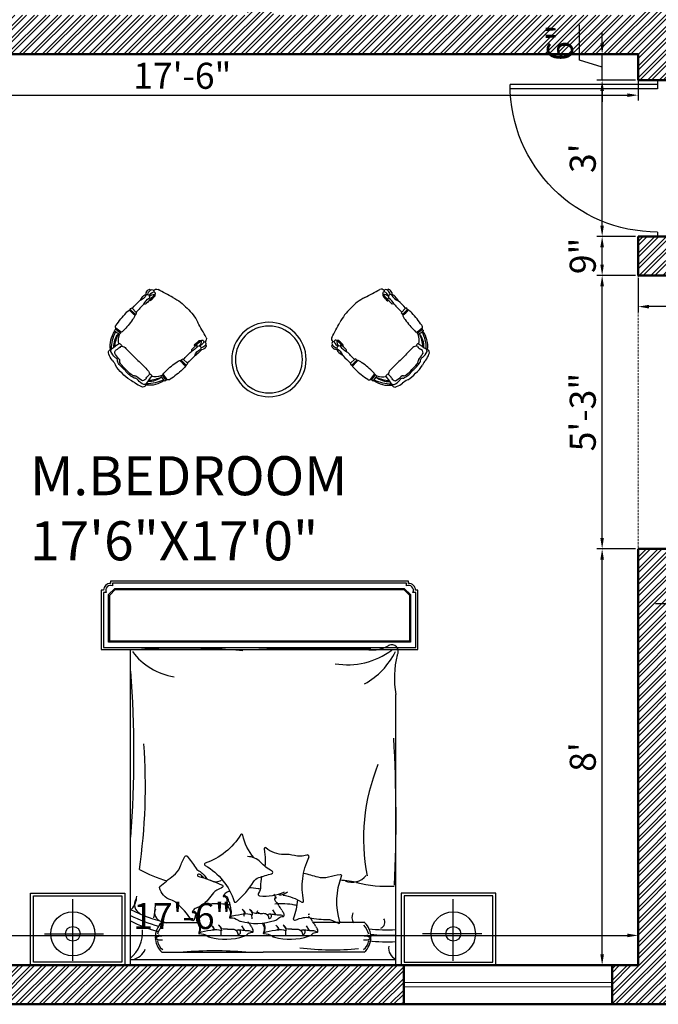
# Model space of a CAD drawing. Units: inches. Extents: x 3590 to 5167, y 65 to 1917.
# Tile 2 of 100: x 3722 to 3869, y 109 to 336. Entities that reach past the tile are written whole.
import ezdxf

# ---------------------------------------------------------------- set-up
doc = ezdxf.new("R2010")
doc.units = ezdxf.units.IN
doc.linetypes.add('DASHED', pattern=[0.75, 0.5, -0.25])
for name, color, linetype, lineweight in [('A-ANNO-DIMS', 2, 'Continuous', 18), ('A-AREA-IDEN', 7, 'Continuous', 18), ('A-DOOR', 3, 'Continuous', 25), ('A-FURN', 21, 'Continuous', 18), ('A-GLAZ', 4, 'Continuous', 18), ('A-WALL', 7, 'Continuous', 50), ('A-WALL-PATT', 251, 'Continuous', 13), ('S-BEAM-OVHD', 7, 'DASHED', 18)]:
    doc.layers.add(name, color=color, linetype=linetype, lineweight=lineweight)
for name, color, linetype in [('FUR', 42, 'Continuous'), ('furn', 7, 'Continuous'), ('HA-FUR', 8, 'Continuous'), ('HA-P', 8, 'Continuous'), ('SAN', 5, 'Continuous'), ('wood', 26, 'Continuous')]:
    doc.layers.add(name, color=color, linetype=linetype)
doc.styles.get("Standard").update_dxf_attribs({"font": 'arial.ttf'})
doc.dimstyles.new('ISO-25', dxfattribs={"dimtxt": 9, "dimasz": 2.5, "dimexe": 1.25, "dimexo": 0.625, "dimtad": 1, "dimdec": 1, "dimlunit": 3, "dimtxsty": 'Standard', "dimcen": 2.5, "dimadec": 0, "dimazin": 0, "dimtfac": 1, "dimtdec": 1, "dimtmove": 0, "dimatfit": 3, "dimfxl": 1, "dimarcsym": 0})

# ---------------------------------------------------------------- blocks, each defined once
blk = doc.blocks.new('D1')
for p, q in [((1, 0), (1, 34)), ((2, 0), (2, 33.99)), ((0, 0), (2, 0)), ((35, 0), (36, 0))]:
    blk.add_line(p, q)
at = {"ltscale": 0.5}
blk.add_arc((1, 0), 34, 0, 90, dxfattribs=at)
blk = doc.blocks.new('*D240')
at = {"layer": 'A-ANNO-DIMS', "color": 0, "lineweight": -2, "transparency": 16777216}
for p, q in [((3654.51, 327.43), (3654.51, 317.35)), ((3864.51, 327.43), (3864.51, 317.35)), ((3657.01, 318.6), (3862.01, 318.6))]:
    blk.add_line(p, q, dxfattribs=at)
at = {"layer": 'A-ANNO-DIMS', "color": 0, "transparency": 16777216}
for points in [[(3657.01, 319.02), (3657.01, 318.18), (3654.51, 318.6)], [(3862.01, 319.02), (3862.01, 318.18), (3864.51, 318.6)]]:
    blk.add_solid(points, dxfattribs=at)
at = {"layer": 'Defpoints', "color": 0, "transparency": 16777216}
for p in [(3654.51, 328.06), (3864.51, 328.06), (3864.51, 318.6)]:
    blk.add_point(p, dxfattribs=at)
at = {"layer": 'A-ANNO-DIMS', "color": 0, "transparency": 16777216, "insert": (3759.51, 322.29), "char_height": 6, "attachment_point": 5}
blk.add_mtext('17\'-6"', dxfattribs=at)
blk = doc.blocks.new('*D194')
at = {"layer": 'A-ANNO-DIMS', "color": 0, "lineweight": -2, "transparency": 16777216}
for p, q in [((3654.51, 118.68), (3654.51, 126.19)), ((3657.01, 124.94), (3862.01, 124.94)), ((3864.51, 118.68), (3864.51, 126.19))]:
    blk.add_line(p, q, dxfattribs=at)
at = {"layer": 'A-ANNO-DIMS', "color": 0, "transparency": 16777216}
for points in [[(3657.01, 125.36), (3657.01, 124.52), (3654.51, 124.94)], [(3862.01, 125.36), (3862.01, 124.52), (3864.51, 124.94)]]:
    blk.add_solid(points, dxfattribs=at)
at = {"layer": 'Defpoints', "color": 0, "transparency": 16777216}
for p in [(3864.51, 124.94), (3654.51, 118.06), (3864.51, 118.06)]:
    blk.add_point(p, dxfattribs=at)
at = {"layer": 'A-ANNO-DIMS', "color": 0, "transparency": 16777216, "insert": (3759.51, 128.63), "char_height": 6, "attachment_point": 5}
blk.add_mtext('17\'-6"', dxfattribs=at)
blk = doc.blocks.new('*D195')
at = {"layer": 'A-ANNO-DIMS', "color": 0, "lineweight": -2, "transparency": 16777216}
for p, q in [((3863.89, 214.06), (3854.98, 214.06)), ((3856.23, 120.56), (3856.23, 211.56)), ((3863.89, 118.06), (3854.98, 118.06))]:
    blk.add_line(p, q, dxfattribs=at)
at = {"layer": 'A-ANNO-DIMS', "color": 0, "transparency": 16777216}
for points in [[(3855.81, 211.56), (3856.64, 211.56), (3856.23, 214.06)], [(3855.81, 120.56), (3856.64, 120.56), (3856.23, 118.06)]]:
    blk.add_solid(points, dxfattribs=at)
at = {"layer": 'Defpoints', "color": 0, "transparency": 16777216}
for p in [(3856.23, 214.06), (3864.51, 214.06), (3864.51, 118.06)]:
    blk.add_point(p, dxfattribs=at)
at = {"layer": 'A-ANNO-DIMS', "color": 0, "transparency": 16777216, "insert": (3852.54, 166.06), "char_height": 6, "attachment_point": 5, "rotation": 90}
blk.add_mtext("8'", dxfattribs=at)
blk = doc.blocks.new('*D196')
at = {"layer": 'A-ANNO-DIMS', "color": 0, "lineweight": -2, "transparency": 16777216}
for p, q in [((3863.89, 277.06), (3854.98, 277.06)), ((3856.23, 216.56), (3856.23, 274.56)), ((3863.89, 214.06), (3854.98, 214.06))]:
    blk.add_line(p, q, dxfattribs=at)
at = {"layer": 'A-ANNO-DIMS', "color": 0, "transparency": 16777216}
for points in [[(3855.81, 274.56), (3856.64, 274.56), (3856.23, 277.06)], [(3855.81, 216.56), (3856.64, 216.56), (3856.23, 214.06)]]:
    blk.add_solid(points, dxfattribs=at)
at = {"layer": 'Defpoints', "color": 0, "transparency": 16777216}
for p in [(3856.23, 277.06), (3864.51, 277.06), (3864.51, 214.06)]:
    blk.add_point(p, dxfattribs=at)
at = {"layer": 'A-ANNO-DIMS', "color": 0, "transparency": 16777216, "insert": (3852.54, 245.56), "char_height": 6, "attachment_point": 5, "rotation": 90}
blk.add_mtext('5\'-3"', dxfattribs=at)
blk = doc.blocks.new('*D197')
at = {"layer": 'A-ANNO-DIMS', "color": 0, "lineweight": -2, "transparency": 16777216}
for p, q in [((3863.89, 286.06), (3854.98, 286.06)), ((3856.23, 279.56), (3856.23, 283.56)), ((3863.89, 277.06), (3854.98, 277.06))]:
    blk.add_line(p, q, dxfattribs=at)
at = {"layer": 'A-ANNO-DIMS', "color": 0, "transparency": 16777216}
for points in [[(3855.81, 283.56), (3856.64, 283.56), (3856.23, 286.06)], [(3855.81, 279.56), (3856.64, 279.56), (3856.23, 277.06)]]:
    blk.add_solid(points, dxfattribs=at)
at = {"layer": 'Defpoints', "color": 0, "transparency": 16777216}
for p in [(3856.23, 286.06), (3864.51, 286.06), (3864.51, 277.06)]:
    blk.add_point(p, dxfattribs=at)
at = {"layer": 'A-ANNO-DIMS', "color": 0, "transparency": 16777216, "insert": (3852.54, 281.56), "char_height": 6, "attachment_point": 5, "rotation": 90}
blk.add_mtext('9"', dxfattribs=at)
blk = doc.blocks.new('*D198')
at = {"layer": 'A-ANNO-DIMS', "color": 0, "lineweight": -2, "transparency": 16777216}
for p, q in [((3863.89, 322.06), (3854.98, 322.06)), ((3856.23, 288.56), (3856.23, 319.56)), ((3863.89, 286.06), (3854.98, 286.06))]:
    blk.add_line(p, q, dxfattribs=at)
at = {"layer": 'A-ANNO-DIMS', "color": 0, "transparency": 16777216}
for points in [[(3855.81, 319.56), (3856.64, 319.56), (3856.23, 322.06)], [(3855.81, 288.56), (3856.64, 288.56), (3856.23, 286.06)]]:
    blk.add_solid(points, dxfattribs=at)
at = {"layer": 'Defpoints', "color": 0, "transparency": 16777216}
for p in [(3856.23, 322.06), (3864.51, 322.06), (3864.51, 286.06)]:
    blk.add_point(p, dxfattribs=at)
at = {"layer": 'A-ANNO-DIMS', "color": 0, "transparency": 16777216, "insert": (3852.54, 304.06), "char_height": 6, "attachment_point": 5, "rotation": 90}
blk.add_mtext("3'", dxfattribs=at)
blk = doc.blocks.new('*D172')
at = {"layer": 'A-ANNO-DIMS', "color": 0, "lineweight": -2, "transparency": 16777216}
for p, q in [((3850.98, 326.64), (3850.98, 334.81)), ((3856.23, 330.56), (3856.23, 333.06)), ((3863.89, 328.06), (3854.98, 328.06)), ((3856.23, 322.06), (3856.23, 328.06)), ((3856.23, 322.06), (3856.23, 328.06)), ((3856.23, 325.06), (3850.98, 326.64)), ((3863.89, 322.06), (3854.98, 322.06)), ((3856.23, 319.56), (3856.23, 317.06))]:
    blk.add_line(p, q, dxfattribs=at)
at = {"layer": 'A-ANNO-DIMS', "color": 0, "transparency": 16777216}
for points in [[(3855.81, 330.56), (3856.64, 330.56), (3856.23, 328.06)], [(3855.81, 319.56), (3856.64, 319.56), (3856.23, 322.06)]]:
    blk.add_solid(points, dxfattribs=at)
at = {"layer": 'Defpoints', "color": 0, "transparency": 16777216}
for p in [(3856.23, 328.06), (3864.51, 328.06), (3864.51, 322.06)]:
    blk.add_point(p, dxfattribs=at)
at = {"layer": 'A-ANNO-DIMS', "color": 0, "transparency": 16777216, "insert": (3847.29, 330.72), "char_height": 6, "attachment_point": 5, "rotation": 90}
blk.add_mtext('6"', dxfattribs=at)
blk = doc.blocks.new('*D173')
at = {"layer": 'A-ANNO-DIMS', "color": 0, "lineweight": -2, "transparency": 16777216}
for p, q in [((3864.51, 276.43), (3864.51, 268.61)), ((3912.51, 276.43), (3912.51, 268.61)), ((3910.01, 269.86), (3867.01, 269.86))]:
    blk.add_line(p, q, dxfattribs=at)
at = {"layer": 'A-ANNO-DIMS', "color": 0, "transparency": 16777216}
for points in [[(3867.01, 270.28), (3867.01, 269.44), (3864.51, 269.86)], [(3910.01, 270.28), (3910.01, 269.44), (3912.51, 269.86)]]:
    blk.add_solid(points, dxfattribs=at)
at = {"layer": 'Defpoints', "color": 0, "transparency": 16777216}
for p in [(3864.51, 277.06), (3912.51, 277.06), (3864.51, 269.86)]:
    blk.add_point(p, dxfattribs=at)
at = {"layer": 'A-ANNO-DIMS', "color": 0, "transparency": 16777216, "insert": (3888.51, 273.49), "char_height": 6, "attachment_point": 5}
blk.add_mtext("4'", dxfattribs=at)
blk = doc.blocks.new('*D175')
at = {"layer": 'A-ANNO-DIMS', "color": 0, "lineweight": -2, "transparency": 16777216}
for p, q in [((3873.51, 204.43), (3873.51, 200.12)), ((3876.51, 204.43), (3876.51, 200.12)), ((3871.01, 201.37), (3868.51, 201.37)), ((3873.51, 201.37), (3876.51, 201.37)), ((3879.01, 201.37), (3889.65, 201.37))]:
    blk.add_line(p, q, dxfattribs=at)
at = {"layer": 'A-ANNO-DIMS', "color": 0, "transparency": 16777216}
for points in [[(3871.01, 201.79), (3871.01, 200.95), (3873.51, 201.37)], [(3879.01, 201.79), (3879.01, 200.95), (3876.51, 201.37)]]:
    blk.add_solid(points, dxfattribs=at)
at = {"layer": 'Defpoints', "color": 0, "transparency": 16777216}
for p in [(3873.51, 205.06), (3876.51, 205.06), (3876.51, 201.37)]:
    blk.add_point(p, dxfattribs=at)
at = {"layer": 'A-ANNO-DIMS', "color": 0, "transparency": 16777216, "insert": (3885.58, 205.06), "char_height": 6, "attachment_point": 5}
blk.add_mtext('3"', dxfattribs=at)
blk = doc.blocks.new('A$C0A42580C')
at = {"layer": 'SAN'}
for p, q in [((0.2873, 0.0301), (0.2873, 0.4484)), ((2.8678, 0.0301), (2.8678, 0.4484)), ((0.0949, 0.2135), (0.4958, 0.2135)), ((3.0601, 0.2135), (2.6592, 0.2135))]:
    blk.add_line(p, q, dxfattribs=at)
for centre, radius in [((0.2873, 0.2135), 0.15), ((2.8678, 0.2135), 0.15), ((0.2873, 0.2135), 0.05), ((2.8678, 0.2135), 0.05)]:
    blk.add_circle(centre, radius, dxfattribs=at)
at = {"layer": 'wood'}
for p, q in [((0.6775, 0.8851), (0.6775, 2.1392)), ((2.4775, 0.8016), (2.4775, 1.838)), ((2.4775, 0), (2.4775, 0.8016)), ((1.5, 0.3423), (1.5016, 0.3142)), ((1.6633, 0.3438), (1.6434, 0.3761)), ((0.888, 0.289), (1.1327, 0.289)), ((1.4538, 0.2362), (1.434, 0.2685)), ((1.8919, 0.2362), (1.8721, 0.2685)), ((2.267, 0.289), (1.9163, 0.289)), ((1.2906, 0.2348), (1.2921, 0.2067)), ((1.7287, 0.2348), (1.7302, 0.2067)), ((0.8909, 0.089), (1.5775, 0.089)), ((2.2642, 0.089), (1.5775, 0.089)), ((0.6775, 0.039), (2.4775, 0.039)), ((0.6775, 0), (2.4775, 0))]:
    blk.add_line(p, q, dxfattribs=at)
blk.add_lwpolyline([(0.6775, 0), (0.6775, 0.8851)], dxfattribs=at)
for points in [[(1.516, 0.7294, -0.128392), (1.4401, 0.8834, 0.70791), (1.427, 0.8863, -0.16964), (1.1848, 0.6919, 0.664036), (1.184, 0.6776, -0.184649), (1.3819, 0.4332, 0.662242), (1.3969, 0.4309, 0.078539), (1.5137, 0.5669, -0.1736), (1.5484, 0.5947, -0.02159), (1.6357, 0.6205, 0.697276), (1.6379, 0.6405, -0.093019), (1.5606, 0.699, 0.216632), (1.4719, 0.7371, -2.511293)], [(1.1211, 0.3454, 0.032543), (1.1095, 0.3091, -0.658965), (1.0917, 0.3063, 0.074753), (0.9887, 0.4234, 0.100988), (0.953, 0.4429, -0.270711), (0.8753, 0.5273, -0.276825), (0.8775, 0.5337, -0.014937), (0.9701, 0.6081, 0.134834), (1.0135, 0.6643, -0.023706), (1.0474, 0.7372, -0.664036), (1.0616, 0.7394, -0.035987), (1.119, 0.6627, 0.118631), (1.1415, 0.6412, -0.132738), (1.1955, 0.5864)], [(1.6795, 0.4818, 0.263265), (1.7191, 0.4839, -0.026108), (1.743, 0.4973, 0.027613), (1.7137, 0.4764, -0.089259), (1.8403, 0.429, 0.662242), (1.8528, 0.4376, -0.162037), (1.8882, 0.732, 0.676499), (1.8733, 0.748, -0.160513), (1.7901, 0.7439, 0.07473), (1.7202, 0.7523, -0.187721), (1.5966, 0.7963, 0.70791), (1.5851, 0.7895, -0.010003), (1.5921, 0.7143, -0.07079), (1.5891, 0.6719, 0.099539)], [(1.1759, 0.5928, 0.013884), (1.1549, 0.6131, 0.174178), (1.1437, 0.6177, 0.104076), (1.1358, 0.6165, 0.389829), (1.1324, 0.6097, 0.296089), (1.1415, 0.6019, -0.036701), (1.1572, 0.5985, -0.040547), (1.3022, 0.543, -0.70791), (1.3021, 0.5296, -0.016811), (1.2631, 0.5085, 0.11866), (1.2414, 0.4904, -0.048791), (1.1649, 0.4055, 0.103757)], [(1.8113, 0.4446, -0.069098), (1.7831, 0.3187, 0.658965), (1.7961, 0.3062, -0.049789), (1.8516, 0.3234, -0.103757), (1.8905, 0.3233, 0.055725), (2.0203, 0.3103, -0.11866), (2.0478, 0.304, 0.016811), (2.0881, 0.2856, 0.70791), (2.0989, 0.2936, -0.16964), (2.1104, 0.604, 0.664036), (2.1001, 0.6139, 0.023706), (2.0214, 0.597, -0.134834), (1.9505, 0.5976, 0.012748), (1.8522, 0.6228)], [(1.5674, 0.601, 0.057807), (1.5606, 0.5339, -0.173425), (1.5457, 0.49, 0.589988), (1.5538, 0.4706, 0.137312), (1.7236, 0.4985, 0.137312)], [(1.3107, 0.4764, 0.145733), (1.3069, 0.4677, 0.488583), (1.3089, 0.4657, -0.012138), (1.3131, 0.4661, -0.125673), (1.3213, 0.4646, -0.750706)], [(1.3153, 0.4751, -0.274893), (1.3379, 0.4529, 0.051436), (1.3468, 0.4293, -0.086628), (1.3532, 0.4078, 0.040196), (1.3593, 0.3772, -0.184744), (1.3556, 0.3344, -2.554464)], [(1.317, 0.4683, -0.060098), (1.3283, 0.4571, -0.16247), (1.3313, 0.4487, 0.120018), (1.3493, 0.3815, -0.060072), (1.3541, 0.3695, -0.13107), (1.3541, 0.3395, -0.024415), (1.3534, 0.3373, 0.070398), (1.3503, 0.3233, 0.528689), (1.3524, 0.3216, -0.069388), (1.3557, 0.3222, -0.158233), (1.4075, 0.3065, 0.085461), (1.4255, 0.2981, 0.147196), (1.6571, 0.3041, 0.10985), (1.6823, 0.3191, -0.179095), (1.7126, 0.3319, -2.318897)], [(1.1013, 0.3688, 0.145733), (1.0975, 0.3601, 0.488583), (1.0995, 0.3581, -0.012138), (1.1036, 0.3585, -0.125673), (1.1119, 0.357, -0.750706)], [(1.1059, 0.3675, -0.274893), (1.1285, 0.3453, 0.051436), (1.1373, 0.3217, -0.086628), (1.1438, 0.3003, 0.040196), (1.1499, 0.2696, -0.184744), (1.1462, 0.2269, -2.554464)], [(1.1076, 0.3607, -0.060098), (1.1189, 0.3495, -0.16247), (1.1219, 0.3411, 0.120018), (1.1399, 0.2739, -0.060072), (1.1447, 0.2619, -0.13107), (1.1447, 0.2319, -0.024415), (1.144, 0.2297, 0.070398), (1.1409, 0.2157, 0.528689), (1.143, 0.2141, -0.069388), (1.1463, 0.2146, -0.158233), (1.1981, 0.1989, 0.085461), (1.2161, 0.1905, 0.147196), (1.4477, 0.1965, 0.10985), (1.4728, 0.2115, -0.179095), (1.5032, 0.2244, -2.318897)], [(1.3509, 0.3219, -0.117141), (1.3688, 0.335, -0.025084), (1.4533, 0.348, 0.033691)], [(1.4359, 0.3803, -0.198519), (1.452, 0.3494, 0.826402), (1.4558, 0.349, 0.095956), (1.4561, 0.3528, 0.242899), (1.4461, 0.3686, -17.523452)], [(1.5447, 0.3525, -0.083557), (1.507, 0.3546, 0.203162), (1.4851, 0.3792, -0.208037), (1.5043, 0.3409, 0.124669), (1.4432, 0.3469, 0.965934)], [(1.5394, 0.3688, 0.145733), (1.5356, 0.3601, 0.488583), (1.5376, 0.3581, -0.012138), (1.5418, 0.3585, -0.125673), (1.55, 0.357, -0.750706)], [(1.5447, 0.3525, -0.008229), (1.5728, 0.3519, 0.033691)], [(1.5728, 0.3519, -0.46905), (1.6152, 0.321, 0.420988), (1.62, 0.3169, 0.857652), (1.6221, 0.3484, 0.548526)], [(1.603, 0.3451, -0.099719), (1.6221, 0.3484, 0.102691)], [(1.6214, 0.3487, -0.010168), (1.6558, 0.3447, 0.033691), (1.6907, 0.3423, -0.220869), (1.7148, 0.3311, -0.288972)], [(1.2265, 0.2728, -0.198519), (1.2426, 0.2418, 0.826402), (1.2463, 0.2415, 0.095956), (1.2467, 0.2452, 0.242899), (1.2366, 0.2611, -17.523452)], [(1.3353, 0.2449, -0.083557), (1.2976, 0.247, 0.203162), (1.2757, 0.2717, -0.208037), (1.2948, 0.2333, 0.124669), (1.2338, 0.2393, 0.965934)], [(1.5721, 0.286, 0.022869), (1.578, 0.2739, -0.060072), (1.5828, 0.2619, -0.13107), (1.5828, 0.2319, -0.024415), (1.5821, 0.2297, 0.070398), (1.579, 0.2157, 0.528689), (1.5811, 0.2141, -0.069388), (1.5844, 0.2146, -0.158233), (1.6362, 0.1989, 0.085461), (1.6542, 0.1905, 0.147196), (1.8858, 0.1965, 0.10985), (1.911, 0.2115, -0.179095), (1.9413, 0.2244, -2.318897)], [(1.5838, 0.2873, 0.023398), (1.588, 0.2696, -0.184744), (1.5843, 0.2269, -2.554464)], [(1.6646, 0.2728, -0.198519), (1.6807, 0.2418, 0.826402), (1.6845, 0.2415, 0.095956), (1.6848, 0.2452, 0.242899), (1.6748, 0.2611, -17.523452)], [(1.7734, 0.2449, -0.083557), (1.7357, 0.247, 0.203162), (1.7138, 0.2717, -0.208037), (1.733, 0.2333, 0.124669), (1.6719, 0.2393, 0.965934)], [(1.1415, 0.2143, -0.117141), (1.1594, 0.2274, -0.025084), (1.2439, 0.2405, 0.033691)], [(1.3353, 0.2449, -0.008229), (1.3633, 0.2443, 0.033691)], [(1.3633, 0.2443, -0.46905), (1.4058, 0.2134, 0.420988), (1.4106, 0.2093, 0.857652), (1.4127, 0.2408, 0.548526)], [(1.3936, 0.2375, -0.099719), (1.4127, 0.2408, 0.102691)], [(1.412, 0.2411, -0.010168), (1.4464, 0.2371, 0.033691), (1.4812, 0.2348, -0.220869), (1.5054, 0.2235, -0.288972)], [(1.5796, 0.2143, -0.117141), (1.5975, 0.2274, -0.025084), (1.682, 0.2405, 0.033691)], [(1.7734, 0.2449, -0.008229), (1.8015, 0.2443, 0.033691)], [(1.8015, 0.2443, -0.46905), (1.8439, 0.2134, 0.420988), (1.8487, 0.2093, 0.857652), (1.8508, 0.2408, 0.548526)], [(1.8317, 0.2375, -0.099719), (1.8508, 0.2408, 0.102691)], [(1.8501, 0.2411, -0.010168), (1.8845, 0.2371, 0.033691), (1.9193, 0.2348, -0.220869), (1.9435, 0.2235, -0.288972)]]:
    blk.add_lwpolyline(points, format="xyb", dxfattribs=at)
for points in [[(0.64, 0), (0, 0), (0, 0.49), (0.64, 0.49)], [(0.62, 0.02), (0.02, 0.02), (0.02, 0.47), (0.62, 0.47)], [(2.515, 0), (3.155, 0), (3.155, 0.49), (2.515, 0.49)], [(2.535, 0.02), (3.135, 0.02), (3.135, 0.47), (2.535, 0.47)]]:
    blk.add_lwpolyline(points, close=True, dxfattribs=at)
for centre, radius, start, end in [((1.0344, -2.14), 4.292, 84.56078, 94.7164), ((2.0208, -11.0786), 13.2288, 88.75549, 92.51133), ((2.1491, 2.5471), 0.5083, 260.65485, 306.44155), ((2.3125, 2.3833), 0.2443, 254.1515, 300.95574), ((2.4501, 2.1309), 0.0445, 324.18954, 118.92203), ((1.0494, 2.4026), 0.4515, 217.47941, 260.35986), ((2.0168, 2.3573), 0.5127, 299.08175, 333.44367), ((3.1371, 1.9502), 0.669, 166.6404, 189.65708), ((-7.0839, 1.4328), 7.7858, 355.84817, 4.15183), ((-7.2439, 0.9937), 9.7233, 357.34474, 3.23068), ((-3.167, 1.2143), 3.9465, 351.77286, 4.18386), ((3.5803, 0.8622), 1.3213, 157.81295, 191.15154), ((1.1611, 1.4181), 0.8768, 241.21362, 254.41879), ((2.181, 0.6859), 0.1221, 247.37754, 321.13165), ((1.2583, 0.6364), 0.0695, 238.58923, 301.92671), ((1.7861, -2.1601), 2.7557, 80.89877, 83.46656), ((2.4192, 1.3819), 0.8461, 255.77539, 273.25587), ((0.5904, 0.4689), 0.13, 317.38218, 359.70393), ((1.3546, 0.4469), 0.0529, 114.21284, 146.15395), ((2.6126, -2.3504), 3.1201, 113.83178, 114.21284), ((1.4714, 0.0722), 0.4528, 80.62397, 88.74059), ((1.4035, -0.3388), 0.8693, 79.71489, 80.62397), ((1.6301, 0.4539), 0.0342, 31.14095, 54.95422), ((1.5664, 0.4154), 0.1086, 24.20989, 31.14095), ((0.7723, 0.4131), 0.0674, 147.68233, 245.79865), ((0.0312, 0.4583), 0.8174, 350.42368, 356.2506), ((2.4032, -2.458), 3.1201, 113.55686, 114.21284), ((1.2046, 0.2912), 0.121, 99.42032, 113.55686), ((1.2774, -0.1478), 0.5659, 95.90379, 99.42032), ((1.2626, -0.005), 0.4223, 88.74059, 95.90379), ((1.2619, -0.0354), 0.4528, 80.62397, 88.74059), ((1.1941, -0.4464), 0.8693, 79.45871, 80.62397), ((1.6709, 0.4489), 0.0156, 131.9623, 212.08127), ((1.6729, 0.4422), 0.0178, 140.41793, 157.63267), ((1.7007, -0.005), 0.4223, 88.74059, 95.90379), ((1.7235, 0.4818), 0.0777, 212.08127, 227.364), ((1.6635, 0.4499), 0.00568, 95.52245, 140.41793), ((1.6627, 0.4587), 0.00309, 275.52245, 24.20989), ((1.6391, 0.3902), 0.0469, 17.32618, 47.364), ((1.7106, 0.4125), 0.028, 197.32618, 226.17302), ((1.7001, -0.0354), 0.4528, 80.62397, 88.74059), ((1.6322, -0.4464), 0.8693, 78.43923, 80.62397), ((1.1611, 1.3191), 1.0568, 242.76671, 257.10398), ((1.1611, 1.3191), 1.0937, 243.75553, 254.4906), ((0.9021, 0.3562), 0.0605, 155.8342, 254.41058), ((1.1452, 0.3394), 0.0529, 114.21284, 146.15395), ((1.4207, 0.3463), 0.0342, 31.14095, 54.95422), ((1.4614, 0.3413), 0.0156, 131.9623, 212.08127), ((1.4635, 0.3347), 0.0178, 140.41793, 157.63267), ((1.4541, 0.3424), 0.00568, 95.52245, 140.41793), ((1.357, 0.3078), 0.1086, 24.20989, 31.14095), ((1.4533, 0.3511), 0.00309, 275.52245, 24.20989), ((1.6431, 0.3422), 0.0695, 26.61764, 46.17302), ((1.8202, 0.431), 0.1287, 206.61764, 215.96192), ((1.6975, 0.3419), 0.023, 350.76434, 35.96192), ((1.7058, 0.3406), 0.0145, 328.02977, 350.76434), ((1.9016, 0.3347), 0.0178, 140.41793, 157.63267), ((1.8922, 0.3424), 0.00568, 95.52245, 140.41793), ((2.2511, 0.3256), 0.071, 155.86842, 211.04513), ((1.1611, 1.2816), 1.0937, 243.75553, 254.38927), ((0.9846, 0.1903), 0.1381, 134.39284, 227.23745), ((0.9986, 0.1735), 0.1427, 136.58239, 164.9725), ((1.5012, 0.305), 0.028, 197.32618, 226.17302), ((1.4337, 0.2347), 0.0695, 26.61764, 46.17302), ((1.715, 0.3349), 0.00379, 207.1817, 328.02977), ((1.9522, 0.3743), 0.0777, 212.08127, 227.364), ((1.8678, 0.2827), 0.0469, 17.32618, 47.364), ((1.9393, 0.305), 0.028, 197.32618, 226.17302), ((1.8718, 0.2347), 0.0695, 26.61764, 46.17302), ((2.1565, 0.1735), 0.1427, 15.0275, 43.41761), ((2.1704, 0.1903), 0.1381, 312.76255, 45.60716), ((2.3616, 0.2915), 0.0419, 290.78583, 35.36309), ((0.5293, 0.2241), 0.2307, 309.63048, 4.27465), ((0.8698, 0.1793), 0.0229, 77.14902, 159.1786), ((1.6108, 0.3235), 0.1287, 206.61764, 215.96192), ((1.5055, 0.2273), 0.00379, 207.1817, 328.02977), ((1.4881, 0.2344), 0.023, 350.76434, 35.96192), ((1.4964, 0.233), 0.0145, 328.02977, 350.76434), ((2.0489, 0.3235), 0.1287, 206.61764, 215.96192), ((1.9436, 0.2273), 0.00379, 207.1817, 328.02977), ((1.9262, 0.2344), 0.023, 350.76434, 35.96192), ((1.9345, 0.233), 0.0145, 328.02977, 350.76434), ((2.2853, 0.1793), 0.0229, 20.8214, 102.85098), ((2.4192, 1.2667), 1.0261, 263.09035, 273.25587), ((2.4192, 1.2667), 1.0629, 263.94374, 273.25587), ((0.8396, 0.185), 0.0112, 314.89662, 45.10338), ((0.8413, 0.1846), 0.0128, 299.47062, 57.44416), ((0.8844, 0.2286), 0.0569, 229.70587, 281.11527), ((0.8802, 0.1371), 0.0592, 81.47786, 123.11925), ((0.9466, 0.1765), 0.0862, 185.53723, 234.68694), ((2.2085, 0.1765), 0.0862, 305.31306, 354.46277), ((2.2706, 0.2286), 0.0569, 258.88473, 310.29413), ((2.2749, 0.1371), 0.0592, 56.88075, 98.52214), ((2.4192, 1.2218), 1.0629, 263.23622, 273.25587), ((2.3138, 0.1846), 0.0128, 122.55584, 240.52938), ((2.3154, 0.185), 0.0112, 134.89662, 225.10338), ((0.6729, 0.151), 0.1135, 279.23824, 338.73819), ((1.2481, -2.5919), 2.6893, 85.4722, 94.5278), ((2.0447, 1.7022), 1.5979, 262.13639, 276.48786), ((2.508, 0.1152), 0.0792, 169.94668, 248.24015)]:
    blk.add_arc(centre, radius, start, end, dxfattribs=at)
blk = doc.blocks.new('A$C623F1DA0')
at = {"layer": 'FUR'}
blk.add_lwpolyline([(0.628, 2.912, 0.414214), (0.562, 2.978), (0.562, 3), (0, 3), (0, 0), (0.562, 0), (0.562, 0.022, 0.414214), (0.628, 0.088), (0.65, 0.088), (0.65, 2.912)], format="xyb", close=True, dxfattribs=at)
at = {"layer": 'HA-FUR'}
blk.add_lwpolyline([(0.6034, 2.892, 0.710288), (0.542, 2.9534), (0.542, 2.98), (0.02, 2.98), (0.02, 0.02), (0.542, 0.02), (0.542, 0.0466, 0.710288), (0.6034, 0.108), (0.63, 0.108), (0.63, 2.892)], format="xyb", close=True, dxfattribs=at)
at = {"layer": 'HA-P'}
for points in [[(0.07, 2.93), (0.5213, 2.93), (0.58, 2.8713), (0.58, 0.1287), (0.5213, 0.07), (0.07, 0.07)], [(0.08, 2.92), (0.5171, 2.92), (0.57, 2.8671), (0.57, 0.1329), (0.5171, 0.08), (0.08, 0.08)]]:
    blk.add_lwpolyline(points, close=True, dxfattribs=at)
blk = doc.blocks.new('CHAIR6')
at = {"layer": 'furn'}
for p, q in [((0.41, 0.26), (0.4094, 0.3185)), ((0.4281, 0.3181), (0.4272, 0.263)), ((0.41, -0.26), (0.4094, -0.3185)), ((0.4281, -0.3181), (0.4272, -0.263))]:
    blk.add_line(p, q, dxfattribs=at)
for centre in [(0.4053, 0.3148), (0.2174, 0.2867), (0.2187, 0.2766), (0.22, 0.2683), (0.2209, 0.2599), (0.2221, 0.2517), (0.2231, 0.2433), (0.4052, 0.3065), (0.4053, 0.2897), (0.4054, 0.2981), (0.4054, 0.2729), (0.4055, 0.2812), (0.4056, 0.2643), (0.2174, -0.2867), (0.2187, -0.2766), (0.22, -0.2683), (0.2209, -0.2599), (0.2221, -0.2517), (0.2231, -0.2433), (0.4052, -0.3065), (0.4053, -0.2897), (0.4053, -0.3148), (0.4054, -0.2981), (0.4054, -0.2729), (0.4055, -0.2812), (0.4056, -0.2643)]:
    blk.add_circle(centre, 0.00425, dxfattribs=at)
for centre, radius, start, end in [((0.3719, -0.3167), 0.6382, 90.6066, 102.05541), ((0.3772, 0.1685), 0.1534, 77.89638, 94.52684), ((3.3638, 0.3149), 2.9628, 179.90105, 181.14792), ((0.4178, 0.2794), 0.04, 75.21702, 102.18253), ((0.5573, 0.1986), 0.1211, 80.56871, 102.58021), ((0.569, 0.3057), 0.0148, 11.93121, 56.71364), ((0.5574, 0.3682), 0.0592, 293.70731, 312.31146), ((0.6147, 0.2731), 0.0542, 72.72663, 108.72189), ((0.6287, 0.3179), 0.00734, 318.72654, 73.20464), ((0.2315, 0.0781), 0.2058, 99.53594, 142.96968), ((0.288, -0.009), 0.2959, 107.467, 135.69066), ((0.2204, 0.0839), 0.1637, 95.98601, 137.80844), ((0.2974, -0.0268), 0.2892, 108.96584, 130.74832), ((0.1998, 0.3299), 0.0425, 267.37882, 299.53851), ((0.5076, 0.3087), 0.3105, 183.92135, 193.66405), ((0.217, 0.2087), 0.0298, 85.88245, 112.38941), ((0.91, 0.35), 0.6998, 184.95819, 189.17441), ((0.2036, 0.356), 0.1186, 277.54736, 281.93488), ((0.2369, 0.2913), 0.0162, 83.97727, 174.0092), ((2.2364, 0.5463), 2.0315, 187.16408, 188.67417), ((0.2433, 0.2647), 0.029, 238.53775, 274.93529), ((0.2506, 0.8795), 0.6438, 269.57373, 280.24813), ((0.357, 0.3514), 0.1057, 274.42127, 300.14813), ((0.4118, 0.3013), 0.0413, 267.60688, 291.9537), ((0.4709, 1.0442), 0.7753, 266.77935, 273.30843), ((0.4807, -0.3094), 0.6241, 87.1388, 94.84242), ((0.5163, 0.348), 0.0344, 262.5365, 295.12391), ((0.5543, 0.4048), 0.1004, 244.96152, 286.92621), ((0.5583, 0.1491), 0.1284, 78.32163, 109.43704), ((0.5171, 0.2599), 0.0105, 7.92951, 98.404), ((0.5475, 0.4175), 0.1574, 262.69111, 279.4279), ((0.5763, 0.2592), 0.00554, 151.0446, 320.63906), ((0.5726, 0.2536), 0.00119, 58.88827, 217.83169), ((0.5864, 0.2986), 0.0481, 252.15364, 277.04405), ((0.5749, 0.272), 0.00992, 261.06044, 17.03518), ((0.6, 0.6108), 0.3491, 266.32513, 275.76594), ((0.5857, 0.2587), 0.00592, 143.235, 315.8485), ((0.5811, 0.2921), 0.0168, 1.95853, 81.75781), ((0.5706, 0.2994), 0.0282, 299.26311, 346.05528), ((0.54, 0.2614), 0.0504, 352.19447, 0.49312), ((0.5958, 0.265), 0.012, 240.91565, 292.3604), ((0.5993, 0.2232), 0.0286, 84.23587, 104.22566), ((0.6205, 0.2416), 0.0492, 62.08685, 124.06689), ((0.5958, 0.2324), 0.05, 38.36456, 93.27362), ((0.6272, 0.2528), 0.0606, 83.33143, 123.59051), ((0.6298, 0.2592), 0.03, 175.25421, 190.14236), ((0.6039, 0.2608), 0.00773, 242.68072, 299.22641), ((0.6055, 0.322), 0.0704, 267.27867, 279.33441), ((0.6233, 0.2599), 0.0167, 173.50236, 200.39748), ((0.6103, 0.2582), 0.0049, 236.84733, 330.71615), ((0.6462, 0.2619), 0.0322, 179.91617, 191.03659), ((0.6177, 0.2574), 0.00347, 207.27606, 12.12043), ((0.6201, 0.2638), 0.0117, 254.38571, 324.07897), ((0.7103, 0.267), 0.0896, 182.99093, 185.70819), ((0.6264, 0.2651), 0.00881, 232.86154, 349.28828), ((0.6327, 0.2954), 0.0177, 352.68742, 85.29917), ((0.6348, 0.276), 0.0126, 270.96281, 46.15927), ((0.6241, 0.3083), 0.0303, 309.85115, 329.87174), ((0.651, 0.2582), 0.0349, 27.02079, 91.1191), ((5.5909, 1.6415), 5.0957, 195.56602, 197.11239), ((0.1754, 0.1139), 0.1594, 153.58586, 173.67646), ((0.0568, 0.1796), 0.0247, 65.10842, 167.8729), ((0.2078, 0.1391), 0.1575, 161.79448, 183.48135), ((0.076, 0.1763), 0.0215, 90.49656, 146.04111), ((0.0747, 0.2065), 0.00875, 210.7256, 277.12246), ((0.0962, 0.1341), 0.0336, 65.79003, 135.37187), ((1.2944, 7.3493), 7.2545, 260.32992, 260.96162), ((0.1315, 0.2333), 0.0718, 252.51235, 277.4747), ((0.1416, 0.1481), 0.0139, 39.59763, 92.78598), ((0.2701, 0.1022), 0.1479, 115.74239, 145.5422), ((0.1013, 0.1754), 0.0542, 340.13538, 9.97368), ((0.2403, 0.0222), 0.2414, 165.22851, 185.28449), ((-0.0992, 0.1308), 0.1161, 336.07618, 0.28835), ((0.2703, 0.0325), 0.2394, 166.65717, 187.80685), ((0.064, 0.0801), 0.0277, 124.74206, 163.83274), ((0.0904, 0.0544), 0.0465, 139.20017, 173.50108), ((0.0085, 0.1198), 0.0432, 336.84052, 13.12552), ((0.0425, 0.1014), 0.0209, 307.26707, 6.28043), ((0.2344, 0.1031), 0.1711, 161.37859, 179.7853), ((0.1123, 0.1263), 0.0505, 352.81567, 37.47081), ((-4.0332, 0.095), 4.1956, 358.70239, 0.34145), ((0.3444, 0.019), 0.396, 357.24911, 18.10814), ((0.4579, 0.0143), 0.4162, 173.74932, 181.97518), ((0.2403, -0.0222), 0.2414, 174.71551, 194.77149), ((0.2703, -0.0325), 0.2394, 172.19315, 193.34283), ((0.4579, -0.0143), 0.4162, 178.02482, 186.25068), ((0.0904, -0.0544), 0.0465, 186.49892, 220.79983), ((-4.0332, -0.095), 4.1956, 359.65855, 1.29761), ((0.3444, -0.019), 0.396, 341.89186, 2.75089), ((-0.0992, -0.1308), 0.1161, 359.71165, 23.92382), ((0.1754, -0.1139), 0.1594, 186.32354, 206.41414), ((0.064, -0.0801), 0.0277, 196.16726, 235.25794), ((0.0085, -0.1198), 0.0432, 346.87448, 23.15948), ((0.2078, -0.1391), 0.1575, 176.51865, 198.20552), ((0.0425, -0.1014), 0.0209, 353.71957, 52.73293), ((0.2344, -0.1031), 0.1711, 180.2147, 198.62141), ((0.0962, -0.1341), 0.0336, 224.62813, 294.20997), ((0.1416, -0.1481), 0.0139, 267.21402, 320.40237), ((0.1123, -0.1263), 0.0505, 322.52919, 7.18433), ((0.1013, -0.1754), 0.0542, 350.02632, 19.86462), ((5.5909, -1.6415), 5.0957, 162.88761, 164.43398), ((0.0568, -0.1796), 0.0247, 192.1271, 294.89158), ((0.076, -0.1763), 0.0215, 213.95889, 269.50344), ((0.0747, -0.2065), 0.00875, 82.87754, 149.2744), ((0.2315, -0.0781), 0.2058, 217.03032, 260.46406), ((1.2944, -7.3493), 7.2545, 99.03838, 99.67008), ((0.288, 0.009), 0.2959, 224.30934, 252.533), ((0.2204, -0.0839), 0.1637, 222.19156, 264.01399), ((0.2974, 0.0268), 0.2892, 229.25168, 251.03416), ((0.1315, -0.2333), 0.0718, 82.5253, 107.48765), ((0.2701, -0.1022), 0.1479, 214.4578, 244.25761), ((0.5076, -0.3087), 0.3105, 166.33595, 176.07865), ((0.217, -0.2087), 0.0298, 247.61059, 274.11755), ((0.2433, -0.2647), 0.029, 85.06471, 121.46225), ((0.2506, -0.8795), 0.6438, 79.75187, 90.42627), ((0.1998, -0.3299), 0.0425, 60.46149, 92.62118), ((0.91, -0.35), 0.6998, 170.82559, 175.04181), ((0.2036, -0.356), 0.1186, 78.06512, 82.45264), ((2.2364, -0.5463), 2.0315, 171.32583, 172.83592), ((0.2369, -0.2913), 0.0162, 185.9908, 276.02273), ((0.3719, 0.3167), 0.6382, 257.94459, 269.3934), ((0.357, -0.3514), 0.1057, 59.85187, 85.57873), ((3.3638, -0.3149), 2.9628, 178.85208, 180.09895), ((0.4118, -0.3013), 0.0413, 68.0463, 92.39312), ((0.4709, -1.0442), 0.7753, 86.69157, 93.22065), ((0.4807, 0.3094), 0.6241, 265.15758, 272.8612), ((0.5543, -0.4048), 0.1004, 73.07379, 115.03848), ((0.5163, -0.348), 0.0344, 64.87609, 97.4635), ((0.5171, -0.2599), 0.0105, 261.596, 352.07049), ((0.5583, -0.1491), 0.1284, 250.56296, 281.67837), ((0.5475, -0.4175), 0.1574, 80.5721, 97.30889), ((0.5573, -0.1986), 0.1211, 257.41979, 279.43129), ((0.5763, -0.2592), 0.00554, 39.36094, 208.9554), ((0.5726, -0.2536), 0.00119, 142.16831, 301.11173), ((0.5864, -0.2986), 0.0481, 82.95595, 107.84636), ((0.5749, -0.272), 0.00992, 342.96482, 98.93956), ((0.569, -0.3057), 0.0148, 303.28636, 348.06879), ((0.6, -0.6108), 0.3491, 84.23406, 93.67487), ((0.5857, -0.2587), 0.00592, 44.1515, 216.765), ((0.5574, -0.3682), 0.0592, 47.68854, 66.29269), ((0.5811, -0.2921), 0.0168, 278.24219, 358.04147), ((0.5706, -0.2994), 0.0282, 13.94472, 60.73689), ((0.5958, -0.265), 0.012, 67.6396, 119.08435), ((0.54, -0.2614), 0.0504, 359.50688, 7.80553), ((0.5993, -0.2232), 0.0286, 255.77434, 275.76413), ((0.5958, -0.2324), 0.05, 266.72638, 321.63544), ((0.6205, -0.2416), 0.0492, 235.93311, 297.91315), ((0.6272, -0.2528), 0.0606, 236.40949, 276.66857), ((0.6298, -0.2592), 0.03, 169.85764, 184.74579), ((0.6039, -0.2608), 0.00773, 60.77359, 117.31928), ((0.6055, -0.322), 0.0704, 80.66559, 92.72133), ((0.6233, -0.2599), 0.0167, 159.60252, 186.49764), ((0.6103, -0.2582), 0.0049, 29.28385, 123.15267), ((0.6462, -0.2619), 0.0322, 168.96341, 180.08383), ((0.6177, -0.2574), 0.00347, 347.87957, 152.72394), ((0.6201, -0.2638), 0.0117, 35.92103, 105.61429), ((0.7103, -0.267), 0.0896, 174.29181, 177.00907), ((0.6264, -0.2651), 0.00881, 10.71172, 127.13846), ((0.6287, -0.3179), 0.00734, 286.79536, 41.27346), ((0.6327, -0.2954), 0.0177, 274.70083, 7.31258), ((0.6348, -0.276), 0.0126, 313.84073, 89.03719), ((0.6241, -0.3083), 0.0303, 30.12826, 50.14885), ((0.651, -0.2582), 0.0349, 268.8809, 332.97921), ((0.3772, -0.1685), 0.1534, 265.47316, 282.10362), ((0.4178, -0.2794), 0.04, 257.81747, 284.78298), ((0.6147, -0.2731), 0.0542, 251.27811, 287.27337)]:
    blk.add_arc(centre, radius, start, end, dxfattribs=at)
blk = doc.blocks.new('A$C78847651')
at = {"layer": 'furn'}
for radius in [0.3, 0.27]:
    blk.add_circle((1.2923, 0.5659), radius, dxfattribs=at)
at = {"layer": 'furn', "rotation": 315}
blk.add_blockref('CHAIR6', (0.1103, 0.6765), dxfattribs=at)
at = {"layer": 'furn', "xscale": -1, "rotation": 44.99999999999991}
blk.add_blockref('CHAIR6', (2.4743, 0.6765), dxfattribs=at)

msp = doc.modelspace()

# ---------------------------------------------------------------- hatches: boundary and pattern name
at = {"layer": 'A-WALL-PATT', "transparency": 33554687}
h = msp.add_hatch(dxfattribs=at)
h.set_pattern_fill('ANSI32', color=256, scale=0.2)
h.set_pattern_definition([(45, (0, -1216.9392), (-1.3470384, 1.3470384), []), (45, (0.898, -1216.9392), (-1.3470384, 1.3470384), [])])
h.paths.add_polyline_path([(3768.51, 589.06), (3645.51, 589.06), (3645.51, 568.06), (3654.51, 568.06), (3654.51, 580.06), (3671.16, 580.06), (3768.51, 580.06)])
h.paths.add_polyline_path([(3909.51, 589.06), (3816.51, 589.06), (3816.51, 580.06), (3864.51, 580.06), (3864.51, 574.06), (3873.51, 574.06), (3873.51, 580.06), (3909.51, 580.06)])
h.paths.add_polyline_path([(4053.51, 589.06), (3969.51, 589.06), (3969.51, 580.06), (4053.51, 580.06)])
h.paths.add_polyline_path([(4215.51, 589.06), (4113.51, 589.06), (4113.51, 580.06), (4206.51, 580.06), (4206.51, 574.06), (4215.51, 574.06)])
h.paths.add_polyline_path([(3654.51, 520.06), (3645.51, 520.06), (3645.51, 403.06), (3654.51, 403.06), (3654.51, 433.06), (3741.51, 433.06), (3741.51, 439.06), (3654.51, 439.06)], flags=17)
h.paths.add_polyline_path([(3873.51, 538.06), (3864.51, 538.06), (3864.51, 439.06), (3771.51, 439.06), (3771.51, 433.06), (3774.51, 433.06), (3774.51, 337.06), (3654.51, 337.06), (3654.51, 367.06), (3645.51, 367.06), (3645.51, 322.06), (3654.51, 322.06), (3654.51, 328.06), (3864.51, 328.06), (3864.51, 322.06), (3873.51, 322.06), (3873.51, 367.06), (3864.51, 367.06), (3864.51, 337.06), (3780.51, 337.06), (3780.51, 433.06), (3864.51, 433.06), (3864.51, 403.06), (3873.51, 403.06)])
h.paths.add_polyline_path([(3654.51, 274.06), (3645.51, 274.06), (3645.51, 109.06), (3810.51, 109.06), (3810.51, 118.06), (3809.96, 118.06), (3654.51, 118.06)])
h.paths.add_polyline_path([(3915.51, 118.06), (3873.51, 118.06), (3873.51, 135.93), (3873.51, 205.06), (3876.51, 205.06), (3876.51, 214.06), (3864.51, 214.06), (3864.51, 118.06), (3858.51, 118.06), (3858.51, 109.06), (3915.51, 109.06)])
h.paths.add_polyline_path([(4028.01, 118.06), (4002.51, 118.06), (4002.51, 286.06), (3981.51, 286.06), (3981.51, 277.06), (3993.51, 277.06), (3993.51, 214.06), (3921.51, 214.06), (3921.51, 277.06), (3933.51, 277.06), (3933.51, 286.06), (3864.51, 286.06), (3864.51, 277.06), (3912.51, 277.06), (3912.51, 214.06), (3906.51, 214.06), (3906.51, 205.06), (3993.51, 205.06), (3993.51, 118.06), (3951.51, 118.06), (3951.51, 109.06), (4028.01, 109.06)])
h.paths.add_polyline_path([(4203.51, 118.06), (4158.51, 118.06), (4158.51, 310.06), (4194.51, 310.06), (4194.51, 319.06), (4149.51, 319.06), (4149.51, 118.06), (4124.01, 118.06), (4124.01, 109.06), (4203.51, 109.06)])
h.paths.add_polyline_path([(4305.51, 349.06), (4296.51, 349.06), (4296.51, 319.06), (4278.64, 319.06), (4260.51, 319.06), (4260.51, 310.06), (4296.51, 310.06), (4296.51, 304.06), (4305.51, 304.06)])
h.paths.add_polyline_path([(4305.51, 256.06), (4296.51, 256.06), (4296.51, 118.06), (4251.51, 118.06), (4251.51, 109.06), (4305.51, 109.06)])
h.paths.add_polyline_path([(4305.51, 460.06), (4215.51, 460.06), (4215.51, 526.06), (4206.51, 526.06), (4206.51, 460.06), (4149.51, 460.06), (4149.51, 451.06), (4296.51, 451.06), (4296.51, 421.06), (4305.51, 421.06)])

# ---------------------------------------------------------------- linework, layer by layer
at = {"layer": 'A-GLAZ'}
for p, q in [((3858.51, 114.06), (3810.51, 114.06)), ((3858.51, 113.06), (3810.51, 113.06))]:
    msp.add_line(p, q, dxfattribs=at)
at = {"layer": 'A-WALL'}
for p, q in [((3864.51, 328.06), (3654.51, 328.06)), ((3864.51, 322.06), (3864.51, 328.06)), ((3873.51, 322.06), (3864.51, 322.06)), ((3933.51, 286.06), (3864.51, 286.06)), ((3864.51, 277.06), (3864.51, 286.06)), ((3912.51, 277.06), (3864.51, 277.06)), ((3876.51, 214.06), (3864.51, 214.06)), ((3864.51, 118.06), (3864.51, 214.06)), ((3864.51, 118.06), (3654.51, 118.06)), ((3810.51, 109.06), (3810.51, 118.06)), ((3858.51, 109.06), (3858.51, 118.06))]:
    msp.add_line(p, q, dxfattribs=at)
msp.add_lwpolyline([(4305.51, 460.06), (4305.51, 109.06), (3645.51, 109.06), (3645.51, 589.06), (4215.51, 589.06)], dxfattribs=at)
at = {"layer": 'S-BEAM-OVHD'}
msp.add_line((3864.51, 277.06), (3864.51, 214.06), dxfattribs=at)

# ---------------------------------------------------------------- block references
at = {"layer": 'A-DOOR', "xscale": -1, "rotation": 90}
msp.add_blockref('D1', (3869.01, 322.06), dxfattribs=at)
at = {"layer": 'A-FURN'}
for name, p, xscale, yscale, zscale, rotation in [('A$C78847651', (3742.51, 273.86), -28.59533479380236, 28.59533479380236, 28.59533479380236, 180), ('A$C623F1DA0', (3813.77, 190.82), 24.31060204424285, 24.31060204424285, 24.31060204424285, 90)]:
    msp.add_blockref(name, p, dxfattribs=dict(at, xscale=xscale, yscale=yscale, zscale=zscale, rotation=rotation))
at = {"layer": 'A-FURN', "xscale": 33.96864568351422, "yscale": 33.96864568351422, "zscale": 33.96864568351422}
msp.add_blockref('A$C0A42580C', (3724.53, 118.06), dxfattribs=at)

# ---------------------------------------------------------------- texts
at = {"layer": 'A-AREA-IDEN', "insert": (3724.44, 235.39), "char_height": 9, "attachment_point": 1}
msp.add_mtext_dynamic_manual_height_columns('{\\fTimes New Roman|b0|i0|c0|p18;M.BEDROOM\\P 17\'6"X17\'0"}', width=67.3508, gutter_width=12.5, heights=[0], dxfattribs=at)

# ---------------------------------------------------------------- dimensions: what is measured, and where the dimension line sits
at = {"layer": 'A-ANNO-DIMS'}
for base, p1, p2, override, picture, middle in [((3856.23, 328.06), (3864.51, 322.06), (3864.51, 328.06), {"dimtxt": 6, "dimclrd": 0, "dimclre": 0, "dimclrt": 0, "dimtmove": 1}, '*D172', (3847.29, 327.26)), ((3856.23, 322.06), (3864.51, 286.06), (3864.51, 322.06), {"dimtxt": 6, "dimclrd": 0, "dimclre": 0, "dimclrt": 0, "dimtmove": 1}, '*D198', (3852.54, 304.06)), ((3856.23, 286.06), (3864.51, 277.06), (3864.51, 286.06), {"dimtxt": 6, "dimclrd": 0, "dimclre": 0, "dimclrt": 0, "dimtmove": 1}, '*D197', (3852.54, 281.56)), ((3856.23, 277.06), (3864.51, 214.06), (3864.51, 277.06), {"dimtxt": 6, "dimclrd": 0, "dimclre": 0, "dimclrt": 0, "dimtmove": 1}, '*D196', (3852.54, 245.56)), ((3856.23, 214.06), (3864.51, 118.06), (3864.51, 214.06), {"dimtxt": 6, "dimclrd": 0, "dimclre": 0, "dimclrt": 0}, '*D195', (3852.54, 166.06))]:
    dim = msp.add_linear_dim(base=base, p1=p1, p2=p2, angle=90, dimstyle='ISO-25', override=override, dxfattribs=at)
    dim.commit()
    dim.dimension.update_dxf_attribs({"geometry": picture, "text_midpoint": middle})
for base, p1, p2, picture, middle in [((3864.51, 318.6), (3654.51, 328.06), (3864.51, 328.06), '*D240', (3759.51, 322.29)), ((3864.51, 269.86), (3912.51, 277.06), (3864.51, 277.06), '*D173', (3888.51, 273.49)), ((3876.51, 201.37), (3873.51, 205.06), (3876.51, 205.06), '*D175', (3885.58, 205.06)), ((3864.51, 124.94), (3654.51, 118.06), (3864.51, 118.06), '*D194', (3759.51, 128.63))]:
    dim = msp.add_linear_dim(base=base, p1=p1, p2=p2, dimstyle='ISO-25', override={"dimtxt": 6, "dimclrd": 0, "dimclre": 0, "dimclrt": 0}, dxfattribs=at)
    dim.commit()
    dim.dimension.update_dxf_attribs({"geometry": picture, "text_midpoint": middle})

doc.saveas('drawing.dxf')
